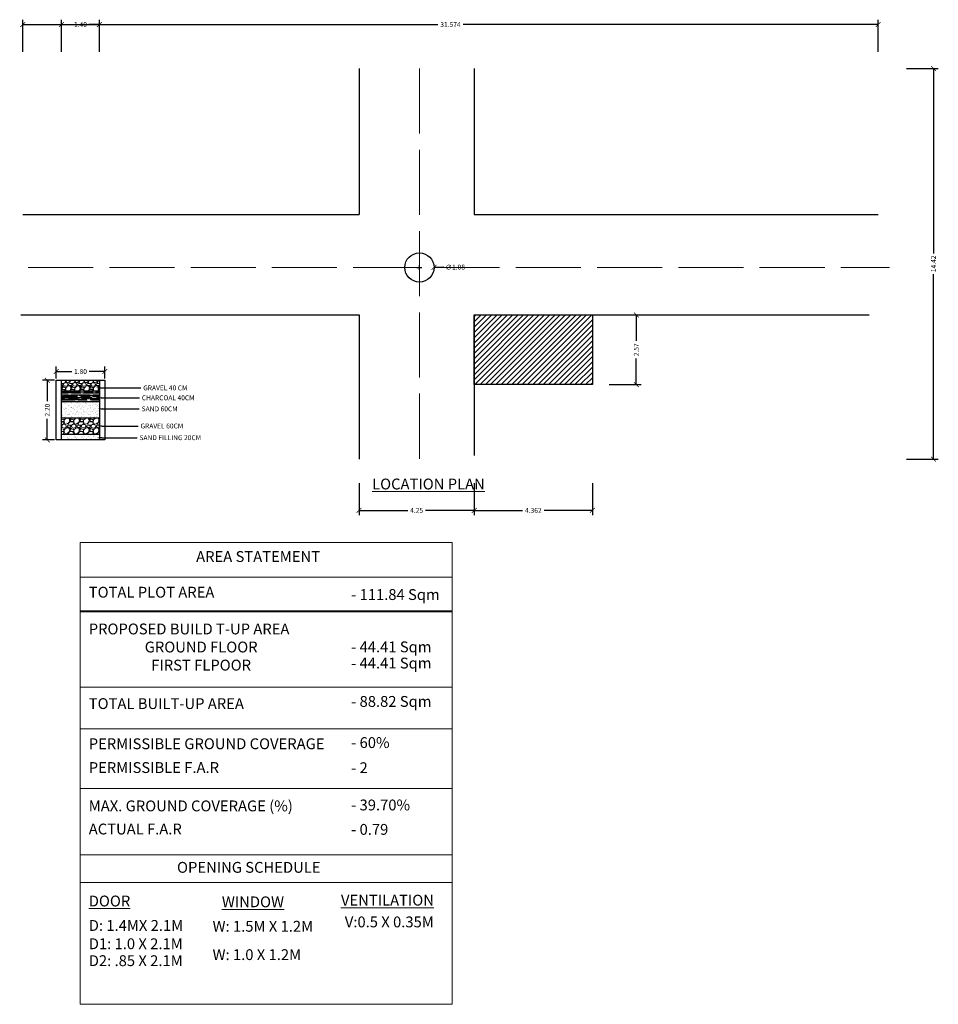
# Model space of a CAD drawing. Units: metres. Extents: x 6.8 to 74, y 0.6 to 37.
# Tile 5 of 5: x 40.1 to 74, y 0.6 to 37. Entities that reach past the tile are written whole.
import ezdxf
from ezdxf import colors
from ezdxf.entities.mleader import LeaderData, LeaderLine
from ezdxf.math import Vec2, Vec3

# ---------------------------------------------------------------- set-up
doc = ezdxf.new("R2010")
doc.units = ezdxf.units.M
doc.header["$LTSCALE"] = 0.2
doc.header["$MEASUREMENT"] = 0
doc.linetypes.add('ACAD_ISO02W100', pattern=[15, 12, -3])
for name, color, linetype, lineweight in [('A-ANNO-DIMS', 2, 'Continuous', 18), ('A-ANNO-SCHD', 7, 'Continuous', 18), ('A-ANNO-TEXT', 7, 'Continuous', 18), ('A-DETL', 7, 'Continuous', 25), ('A-DETL-PATT', 252, 'Continuous', 13), ('A-SCHD-TEXT', 7, 'Continuous', 18), ('C-PROP', 3, 'Continuous', 30), ('C-ROAD', 7, 'Continuous', 25), ('C-ROAD-CNTR', 1, 'ACAD_ISO02W100', 13), ('C-SITE-PATT', 252, 'Continuous', 13)]:
    doc.layers.add(name, color=color, linetype=linetype, lineweight=lineweight)
doc.styles.get("Standard").update_dxf_attribs({"font": 'arial.ttf'})
doc.dimstyles.get("Standard").update_dxf_attribs({"dimtxt": 0.18, "dimasz": 0.18, "dimexe": 0.18, "dimexo": 0.0625, "dimgap": 0.09, "dimtad": 0, "dimzin": 0, "dimdsep": 46, "dimtxsty": 'Standard', "dimblk": 'ARCHTICK', "dimcen": 0.09, "dimadec": 0, "dimazin": 0, "dimtfac": 1, "dimtofl": 0, "dimtmove": 0, "dimatfit": 3, "dimfxl": 1, "dimfxlon": 1, "dimtolj": 1, "dimtzin": 0, "dimarcsym": 0})
pattern_1 = [(37.5, (-6.10384, 6.83686), (-0.00548042, 0.16763367), [0, -0.13224, 0, -0.1479, 0, -0.141375]), (7.5, (-6.10384, 6.83686), (0.1539706, 0.2455267), [0, -0.07134, 0, -0.11919, 0, -0.045675]), (327.5, (-6.21085, 6.83686), (0.27093034, 0.00049234), [0, -0.0435, 0, -0.1566, 0, -0.20445]), (317.5, (-6.21085, 6.83686), (0.261533, 0.0763578), [0, -0.02175, 0, -0.10266, 0, -0.11745])]

# ---------------------------------------------------------------- blocks, each defined once
blk = doc.blocks.new('_ArchTick')
at = {"color": 0, "linetype": 'ByBlock', "const_width": 0.15}
blk.add_lwpolyline([(-0.5, -0.5), (0.5, 0.5)], dxfattribs=at)
blk = doc.blocks.new('*D14')
at = {"layer": 'A-ANNO-DIMS', "color": 0, "lineweight": -2, "ltscale": 0.9, "transparency": 16777216}
for p, q in [((41.484, 23.715), (41.484, 24.158)), ((43.284, 23.715), (43.284, 24.158)), ((41.484, 23.978), (42.069, 23.978)), ((43.284, 23.978), (42.699, 23.978))]:
    blk.add_line(p, q, dxfattribs=at)
at = {"layer": 'Defpoints', "color": 0, "ltscale": 0.9, "transparency": 16777216}
for p in [(41.484, 23.653), (43.284, 23.978), (43.284, 23.653)]:
    blk.add_point(p, dxfattribs=at)
at = {"layer": 'A-ANNO-DIMS', "color": 0, "lineweight": -2, "ltscale": 0.9, "transparency": 16777216, "xscale": 0.18, "yscale": 0.18, "zscale": 0.18, "rotation": 180}
blk.add_blockref('_ArchTick', (41.484, 23.978), dxfattribs=at)
at = {"layer": 'A-ANNO-DIMS', "color": 0, "lineweight": -2, "ltscale": 0.9, "transparency": 16777216, "xscale": 0.18, "yscale": 0.18, "zscale": 0.18}
blk.add_blockref('_ArchTick', (43.284, 23.978), dxfattribs=at)
at = {"layer": 'A-ANNO-DIMS', "color": 0, "ltscale": 0.9, "transparency": 16777216, "insert": (42.384, 23.978), "char_height": 0.18, "attachment_point": 5}
blk.add_mtext('\\A1;1.80', dxfattribs=at)
blk = doc.blocks.new('*D15')
at = {"layer": 'A-ANNO-DIMS', "color": 0, "lineweight": -2, "ltscale": 0.9, "transparency": 16777216}
for p, q in [((41.421, 23.653), (40.981, 23.653)), ((41.161, 23.653), (41.161, 22.878)), ((41.161, 21.453), (41.161, 22.228)), ((41.421, 21.453), (40.981, 21.453))]:
    blk.add_line(p, q, dxfattribs=at)
at = {"layer": 'Defpoints', "color": 0, "ltscale": 0.9, "transparency": 16777216}
for p in [(41.484, 23.653), (41.161, 21.453), (41.484, 21.453)]:
    blk.add_point(p, dxfattribs=at)
at = {"layer": 'A-ANNO-DIMS', "color": 0, "lineweight": -2, "ltscale": 0.9, "transparency": 16777216, "xscale": 0.18, "yscale": 0.18, "zscale": 0.18}
for p, rotation in [((41.161, 23.653), 90), ((41.161, 21.453), 270)]:
    blk.add_blockref('_ArchTick', p, dxfattribs=dict(at, rotation=rotation))
at = {"layer": 'A-ANNO-DIMS', "color": 0, "ltscale": 0.9, "transparency": 16777216, "insert": (41.161, 22.553), "char_height": 0.18, "attachment_point": 5, "rotation": 90}
blk.add_mtext('\\A1;2.20', dxfattribs=at)
blk = doc.blocks.new('*D60')
at = {"layer": 'A-ANNO-DIMS', "color": 0, "lineweight": -2, "ltscale": 0.9, "transparency": 16777216}
for p, q in [((52.667, 19.852), (52.667, 18.672)), ((56.917, 19.852), (56.917, 18.672)), ((52.667, 18.852), (54.464, 18.852)), ((56.917, 18.852), (55.12, 18.852))]:
    blk.add_line(p, q, dxfattribs=at)
at = {"layer": 'Defpoints', "color": 0, "ltscale": 0.9, "transparency": 16777216}
for p in [(52.667, 26.063), (56.917, 26.063), (56.917, 18.852)]:
    blk.add_point(p, dxfattribs=at)
at = {"layer": 'A-ANNO-DIMS', "color": 0, "lineweight": -2, "ltscale": 0.9, "transparency": 16777216, "xscale": 0.18, "yscale": 0.18, "zscale": 0.18, "rotation": 180}
blk.add_blockref('_ArchTick', (52.667, 18.852), dxfattribs=at)
at = {"layer": 'A-ANNO-DIMS', "color": 0, "lineweight": -2, "ltscale": 0.9, "transparency": 16777216, "xscale": 0.18, "yscale": 0.18, "zscale": 0.18}
blk.add_blockref('_ArchTick', (56.917, 18.852), dxfattribs=at)
at = {"layer": 'A-ANNO-DIMS', "color": 0, "ltscale": 0.9, "transparency": 16777216, "insert": (54.792, 18.852), "char_height": 0.18, "attachment_point": 5}
blk.add_mtext('\\A1;4.25', dxfattribs=at)
blk = doc.blocks.new('*D61')
at = {"layer": 'A-ANNO-DIMS', "color": 0, "lineweight": -2, "ltscale": 0.9, "transparency": 16777216}
for p, q in [((39.567, 29.769), (38.387, 29.769)), ((38.567, 29.769), (38.567, 28.31)), ((38.567, 26.063), (38.567, 27.523)), ((39.567, 26.063), (38.387, 26.063))]:
    blk.add_line(p, q, dxfattribs=at)
at = {"layer": 'Defpoints', "color": 0, "ltscale": 0.9, "transparency": 16777216}
for p in [(38.567, 29.769), (52.667, 29.769), (52.667, 26.063)]:
    blk.add_point(p, dxfattribs=at)
at = {"layer": 'A-ANNO-DIMS', "color": 0, "lineweight": -2, "ltscale": 0.9, "transparency": 16777216, "xscale": 0.18, "yscale": 0.18, "zscale": 0.18}
for p, rotation in [((38.567, 29.769), 90), ((38.567, 26.063), 270)]:
    blk.add_blockref('_ArchTick', p, dxfattribs=dict(at, rotation=rotation))
at = {"layer": 'A-ANNO-DIMS', "color": 0, "ltscale": 0.9, "transparency": 16777216, "insert": (38.567, 27.916), "char_height": 0.18, "attachment_point": 5, "rotation": 90}
blk.add_mtext('\\A1;3.706', dxfattribs=at)
blk = doc.blocks.new('*D62')
at = {"layer": 'A-ANNO-DIMS', "color": 0, "lineweight": -2, "ltscale": 0.9, "transparency": 16777216}
for p, q in [((56.917, 19.852), (56.917, 18.672)), ((61.279, 19.852), (61.279, 18.672)), ((56.917, 18.852), (58.702, 18.852)), ((61.279, 18.852), (59.495, 18.852))]:
    blk.add_line(p, q, dxfattribs=at)
at = {"layer": 'Defpoints', "color": 0, "ltscale": 0.9, "transparency": 16777216}
for p in [(56.917, 23.493), (61.279, 23.493), (61.279, 18.852)]:
    blk.add_point(p, dxfattribs=at)
at = {"layer": 'A-ANNO-DIMS', "color": 0, "lineweight": -2, "ltscale": 0.9, "transparency": 16777216, "xscale": 0.18, "yscale": 0.18, "zscale": 0.18, "rotation": 180}
blk.add_blockref('_ArchTick', (56.917, 18.852), dxfattribs=at)
at = {"layer": 'A-ANNO-DIMS', "color": 0, "lineweight": -2, "ltscale": 0.9, "transparency": 16777216, "xscale": 0.18, "yscale": 0.18, "zscale": 0.18}
blk.add_blockref('_ArchTick', (61.279, 18.852), dxfattribs=at)
at = {"layer": 'A-ANNO-DIMS', "color": 0, "ltscale": 0.9, "transparency": 16777216, "insert": (59.098, 18.852), "char_height": 0.18, "attachment_point": 5}
blk.add_mtext('\\A1;4.362', dxfattribs=at)
blk = doc.blocks.new('*D63')
at = {"layer": 'A-ANNO-DIMS', "color": 0, "lineweight": -2, "ltscale": 0.9, "transparency": 16777216}
for p, q in [((61.898, 26.063), (63.078, 26.063)), ((62.898, 26.063), (62.898, 25.103)), ((62.898, 23.493), (62.898, 24.453)), ((61.898, 23.493), (63.078, 23.493))]:
    blk.add_line(p, q, dxfattribs=at)
at = {"layer": 'Defpoints', "color": 0, "ltscale": 0.9, "transparency": 16777216}
for p in [(61.279, 26.063), (61.279, 23.493), (62.898, 23.493)]:
    blk.add_point(p, dxfattribs=at)
at = {"layer": 'A-ANNO-DIMS', "color": 0, "lineweight": -2, "ltscale": 0.9, "transparency": 16777216, "xscale": 0.18, "yscale": 0.18, "zscale": 0.18}
for p, rotation in [((62.898, 26.063), 90), ((62.898, 23.493), 270)]:
    blk.add_blockref('_ArchTick', p, dxfattribs=dict(at, rotation=rotation))
at = {"layer": 'A-ANNO-DIMS', "color": 0, "ltscale": 0.9, "transparency": 16777216, "insert": (62.898, 24.778), "char_height": 0.18, "attachment_point": 5, "rotation": 90}
blk.add_mtext('\\A1;2.57', dxfattribs=at)
blk = doc.blocks.new('*D64')
at = {"layer": 'A-ANNO-DIMS', "color": 0, "lineweight": -2, "ltscale": 0.9, "transparency": 16777216}
for p, q in [((41.683909, 35.779105), (41.683909, 36.959105)), ((41.683909, 36.779105), (42.068909, 36.779105)), ((43.083909, 36.779105), (42.698909, 36.779105)), ((43.083909, 35.779105), (43.083909, 36.959105))]:
    blk.add_line(p, q, dxfattribs=at)
at = {"layer": 'Defpoints', "color": 0, "ltscale": 0.9, "transparency": 16777216}
for p in [(43.083909, 36.779105), (41.683909, 23.652882), (43.083909, 23.652882)]:
    blk.add_point(p, dxfattribs=at)
at = {"layer": 'A-ANNO-DIMS', "color": 0, "lineweight": -2, "ltscale": 0.9, "transparency": 16777216, "xscale": 0.18, "yscale": 0.18, "zscale": 0.18, "rotation": 180}
blk.add_blockref('_ArchTick', (41.683909, 36.779105), dxfattribs=at)
at = {"layer": 'A-ANNO-DIMS', "color": 0, "lineweight": -2, "ltscale": 0.9, "transparency": 16777216, "xscale": 0.18, "yscale": 0.18, "zscale": 0.18}
blk.add_blockref('_ArchTick', (43.083909, 36.779105), dxfattribs=at)
at = {"layer": 'A-ANNO-DIMS', "color": 0, "ltscale": 0.9, "transparency": 16777216, "insert": (42.383909, 36.779105), "char_height": 0.18, "attachment_point": 5}
blk.add_mtext('\\A1;1.40', dxfattribs=at)
blk = doc.blocks.new('*D75')
at = {"layer": 'A-ANNO-DIMS', "color": 0, "lineweight": -2, "ltscale": 0.9, "transparency": 16777216}
for p, q in [((40.253, 35.779), (40.253, 36.959)), ((40.253, 36.779), (55.577, 36.779)), ((71.827, 36.779), (56.504, 36.779)), ((71.827, 35.779), (71.827, 36.959))]:
    blk.add_line(p, q, dxfattribs=at)
at = {"layer": 'Defpoints', "color": 0, "ltscale": 0.9, "transparency": 16777216}
for p in [(71.827, 36.779), (40.253, 29.769), (71.827, 29.769)]:
    blk.add_point(p, dxfattribs=at)
at = {"layer": 'A-ANNO-DIMS', "color": 0, "lineweight": -2, "ltscale": 0.9, "transparency": 16777216, "xscale": 0.18, "yscale": 0.18, "zscale": 0.18, "rotation": 180}
blk.add_blockref('_ArchTick', (40.253, 36.779), dxfattribs=at)
at = {"layer": 'A-ANNO-DIMS', "color": 0, "lineweight": -2, "ltscale": 0.9, "transparency": 16777216, "xscale": 0.18, "yscale": 0.18, "zscale": 0.18}
blk.add_blockref('_ArchTick', (71.827, 36.779), dxfattribs=at)
at = {"layer": 'A-ANNO-DIMS', "color": 0, "ltscale": 0.9, "transparency": 16777216, "insert": (56.04, 36.779), "char_height": 0.18, "attachment_point": 5}
blk.add_mtext('\\A1;31.574', dxfattribs=at)
blk = doc.blocks.new('*D76')
at = {"layer": 'A-ANNO-DIMS', "color": 0, "lineweight": -2, "ltscale": 0.9, "transparency": 16777216}
for p, q in [((72.866, 35.16), (74.046, 35.16)), ((73.866, 35.16), (73.866, 28.334)), ((73.866, 20.74), (73.866, 27.566)), ((72.866, 20.74), (74.046, 20.74))]:
    blk.add_line(p, q, dxfattribs=at)
at = {"layer": 'Defpoints', "color": 0, "ltscale": 0.9, "transparency": 16777216}
for p in [(52.667, 35.16), (73.866, 35.16), (52.667, 20.74)]:
    blk.add_point(p, dxfattribs=at)
at = {"layer": 'A-ANNO-DIMS', "color": 0, "lineweight": -2, "ltscale": 0.9, "transparency": 16777216, "xscale": 0.18, "yscale": 0.18, "zscale": 0.18}
for p, rotation in [((73.866, 35.16), 90), ((73.866, 20.74), 270)]:
    blk.add_blockref('_ArchTick', p, dxfattribs=dict(at, rotation=rotation))
at = {"layer": 'A-ANNO-DIMS', "color": 0, "ltscale": 0.9, "transparency": 16777216, "insert": (73.866, 27.95), "char_height": 0.18, "attachment_point": 5, "rotation": 90}
blk.add_mtext('\\A1;14.42', dxfattribs=at)
blk = doc.blocks.new('*D77')
at = {"layer": 'A-ANNO-DIMS', "color": 0, "lineweight": -2, "ltscale": 0.9, "transparency": 16777216}
for p, q in [((54.803, 27.815), (54.983, 27.815)), ((54.893, 27.725), (54.893, 27.905)), ((55.793, 27.823), (55.433, 27.82))]:
    blk.add_line(p, q, dxfattribs=at)
at = {"layer": 'Defpoints', "color": 0, "ltscale": 0.9, "transparency": 16777216}
for p in [(54.354, 27.811), (55.433, 27.82)]:
    blk.add_point(p, dxfattribs=at)
at = {"layer": 'A-ANNO-DIMS', "color": 0, "lineweight": -2, "ltscale": 0.9, "transparency": 16777216, "xscale": 0.18, "yscale": 0.18, "zscale": 0.18, "rotation": 180.5010629486621}
blk.add_blockref('_ArchTick', (55.433, 27.82), dxfattribs=at)
at = {"layer": 'A-ANNO-DIMS', "color": 0, "ltscale": 0.9, "transparency": 16777216, "insert": (56.215, 27.827), "char_height": 0.18, "attachment_point": 5, "rotation": 0.5011}
blk.add_mtext('\\A1;∅1.08', dxfattribs=at)

msp = doc.modelspace()

# ---------------------------------------------------------------- hatches: boundary and pattern name
at = {"layer": 'A-DETL-PATT', "ltscale": 0.9}
h = msp.add_hatch(dxfattribs=at)
h.set_pattern_fill('GRAVEL', color=256, scale=0.34)
h.set_pattern_definition([(228.01279, (-5.85904, 7.176862), (-2.72, -3.06), [0.0457422, -4.52849]), (184.96974, (-5.88964, 7.142862), (4.08, 0.34), [0.0784951, -7.7710144]), (132.510447, (-5.96784, 7.136062), (3.4, -3.74), [0.055348, -5.479451]), (267.27369, (-6.10044, 7.051062), (0.34, 6.8), [0.071481, -7.0766097]), (292.833654, (-6.10384, 6.979662), (-1.7, 4.08), [0.0700927, -6.9391869]), (357.27369, (-6.07664, 6.915062), (-6.8, 0.34), [0.071481, -7.0766097]), (37.69424, (-6.00524, 6.911662), (-4.42, -3.4), [0.0945299, -9.3584485]), (72.255328, (-5.93044, 6.969462), (2.38, 7.48), [0.089246, -8.8353493]), (121.429566, (-5.90324, 7.054462), (-2.72, 4.42), [0.071723, -7.1005849]), (175.23636, (-5.94064, 7.115662), (3.74, -0.34), [0.0818829, -4.0122593]), (222.397438, (-6.02224, 7.122462), (-4.08, -3.74), [0.1058923, -10.4833475]), (138.814075, (-5.76384, 7.04766), (-2.38, 2.04), [0.0361423, -3.5781072]), (171.469234, (-5.79104, 7.071462), (4.42, -0.68), [0.0687606, -6.8073139]), (225, (-5.85904, 7.08166), (0, -0.34), [0.0480831, -0.4327495]), (203.19859, (-5.88284, 7.12246), (1.7, 0.68), [0.0258937, -2.5634691]), (291.80141, (-5.90664, 7.11226), (-0.34, 1.02), [0.036619, -1.794337]), (30.96376, (-5.89304, 7.07826), (1.02, 0.68), [0.0594759, -1.9230478]), (161.56505, (-5.84204, 7.10886), (0.68, -0.34), [0.043007, -1.0321675]), (16.38954, (-6.10384, 7.112262), (3.4, 1.02), [0.060248, -5.9645673]), (70.346176, (-6.04604, 7.129262), (-1.36, -3.74), [0.0505447, -5.0039186]), (293.19859, (-5.84204, 7.17686), (-0.68, 1.7), [0.051787, -2.5375758]), (343.61046, (-5.82164, 7.129262), (-3.4, 1.02), [0.060248, -5.9645673]), (339.443955, (-6.10384, 6.90146), (-1.7, 0.68), [0.0580992, -2.846862]), (294.77514, (-6.04944, 6.881062), (-1.7, 3.74), [0.0486805, -4.8193786]), (66.80141, (-5.83864, 6.83686), (0.68, 1.7), [0.051787, -2.5375758]), (17.354025, (-5.81824, 6.884462), (-4.42, -1.36), [0.0569945, -5.642444]), (69.443955, (-6.00524, 6.83686), (-0.68, -1.7), [0.0290496, -2.8759117]), (101.30993, (-5.85904, 6.83686), (-0.34, 1.36), [0.0173366, -1.71633]), (165.96376, (-5.86244, 6.85386), (1.02, -0.34), [0.0700927, -1.3317632]), (186.009006, (-5.93044, 6.870862), (3.4, 0.34), [0.064957, -6.4307339]), (303.69007, (-5.89304, 7.04766), (-0.34, 0.68), [0.0490355, -1.176852]), (353.157227, (-5.86584, 7.006862), (5.78, -0.68), [0.08561, -8.4753713]), (60.945396, (-5.78084, 6.99666), (-1.36, -2.38), [0.035005, -3.4655092]), (90, (-5.76384, 7.02726), (-0.34, 0.34), [0.0204, -0.3196]), (120.256437, (-5.93724, 6.881062), (1.36, -2.38), [0.0472342, -4.6761968]), (48.01279, (-5.96104, 6.921862), (2.72, 3.06), [0.0914845, -4.4827477]), (0, (-5.89984, 6.98986), (0.34, 0.34), [0.0884, -0.2516]), (325.304846, (-5.81144, 6.989862), (3.4, -2.38), [0.0537588, -5.3221133]), (254.0546, (-5.76724, 6.95926), (-0.34, -1.36), [0.0495047, -2.4257327]), (207.645975, (-5.78084, 6.911662), (-6.46, -3.4), [0.0806021, -7.9796212]), (175.42608, (-5.85224, 6.874262), (-4.42, 0.34), [0.0852717, -8.441885])])
h.paths.add_polyline_path([(41.6839, 23.6529), (41.6839, 23.2529), (43.0839, 23.2529), (43.0839, 23.6529)])
h = msp.add_hatch(dxfattribs=at)
h.set_pattern_fill('AR-RROOF', color=256, scale=0.087)
h.set_pattern_definition([(0, (-6.10384, 6.83686), (0.1914, 0.087), [1.305, -0.174, 0.435, -0.087]), (0, (-5.98813, 6.88036), (-0.087, 0.11571), [0.261, -0.02871, 0.522, -0.06525]), (0, (-6.06034, 6.91081), (0.4524, 0.05829), [0.696, -0.1218, 0.348, -0.087])])
h.paths.add_polyline_path([(43.0839, 22.8529), (43.0839, 23.2529), (41.6839, 23.2529), (41.6839, 22.8529)])
h = msp.add_hatch(dxfattribs=at)
h.set_pattern_fill('AR-SAND', color=256, scale=0.087)
h.set_pattern_definition(pattern_1)
h.paths.add_polyline_path([(41.6839, 22.8529), (41.6839, 22.2529), (43.0839, 22.2529), (43.0839, 22.8529)])
h = msp.add_hatch(dxfattribs=at)
h.set_pattern_fill('GRAVEL', color=256, scale=0.36)
h.set_pattern_definition([(228.01279, (-5.84464, 7.196862), (-2.88, -3.24), [0.048433, -4.7948717]), (184.96974, (-5.87704, 7.160862), (4.32, 0.36), [0.0831125, -8.228133]), (132.510447, (-5.95984, 7.153662), (3.6, -3.96), [0.0586037, -5.8017717]), (267.27369, (-6.10024, 7.063662), (0.36, 7.2), [0.0756857, -7.492881]), (292.833654, (-6.10384, 6.988062), (-1.8, 4.32), [0.0742158, -7.3473743]), (357.27369, (-6.07504, 6.919662), (-7.2, 0.36), [0.0756857, -7.492881]), (37.69424, (-5.99944, 6.916062), (-4.68, -3.6), [0.1000904, -9.9089455]), (72.255328, (-5.92024, 6.977262), (2.52, 7.92), [0.0944957, -9.3550757]), (121.429566, (-5.89144, 7.067262), (-2.88, 4.68), [0.075942, -7.5182663]), (175.23636, (-5.93104, 7.132062), (3.96, -0.36), [0.0866995, -4.2482745]), (222.397438, (-6.01744, 7.139262), (-4.32, -3.96), [0.1121213, -11.100015]), (138.814075, (-5.74384, 7.06006), (-2.52, 2.16), [0.0382684, -3.7885841]), (171.469234, (-5.77264, 7.085262), (4.68, -0.72), [0.0728053, -7.207744]), (225, (-5.84464, 7.09606), (0, -0.36), [0.0509116, -0.4582053]), (203.19859, (-5.86984, 7.13926), (1.8, 0.72), [0.027417, -2.7142614]), (291.80141, (-5.89504, 7.12846), (-0.36, 1.08), [0.038773, -1.8998863]), (30.96376, (-5.88064, 7.09246), (1.08, 0.72), [0.0629744, -2.0361682]), (161.56505, (-5.82664, 7.12486), (0.72, -0.36), [0.0455368, -1.0928832]), (16.38954, (-6.10384, 7.128462), (3.6, 1.08), [0.063792, -6.3154243]), (70.346176, (-6.04264, 7.146462), (-1.44, -3.96), [0.053518, -5.2982668]), (293.19859, (-5.82664, 7.19686), (-0.72, 1.8), [0.0548334, -2.686845]), (343.61046, (-5.80504, 7.146462), (-3.6, 1.08), [0.063792, -6.3154243]), (339.443955, (-6.10384, 6.90526), (-1.8, 0.72), [0.0615168, -3.0143245]), (294.77514, (-6.04624, 6.883662), (-1.8, 3.96), [0.051544, -5.1028715]), (66.80141, (-5.82304, 6.83686), (0.72, 1.8), [0.0548334, -2.686845]), (17.354025, (-5.80144, 6.887262), (-4.68, -1.44), [0.0603472, -5.9743525]), (69.443955, (-5.99944, 6.83686), (-0.72, -1.8), [0.0307584, -3.045083]), (101.30993, (-5.84464, 6.83686), (-0.36, 1.44), [0.0183564, -1.8172906]), (165.96376, (-5.84824, 6.85486), (1.08, -0.36), [0.0742158, -1.4101022]), (186.009006, (-5.92024, 6.872862), (3.6, 0.36), [0.068778, -6.8090123]), (303.69007, (-5.88064, 7.06006), (-0.36, 0.72), [0.05192, -1.2460785]), (353.157227, (-5.85184, 7.016862), (6.12, -0.72), [0.0906458, -8.9739225]), (60.945396, (-5.76184, 7.00606), (-1.44, -2.52), [0.0370642, -3.6693627]), (90, (-5.74384, 7.03846), (-0.36, 0.36), [0.0216, -0.3384]), (120.25644, (-5.92744, 6.883662), (1.44, -2.52), [0.0500126, -4.9512672]), (48.01279, (-5.95264, 6.926862), (2.88, 3.24), [0.096866, -4.7464387]), (0, (-5.88784, 6.99886), (0.36, 0.36), [0.0936, -0.2664]), (325.304846, (-5.79424, 6.998862), (3.6, -2.52), [0.056921, -5.6351787]), (254.0546, (-5.74744, 6.96646), (-0.36, -1.44), [0.0524167, -2.5684228]), (207.645975, (-5.76184, 6.916062), (-6.84, -3.6), [0.0853434, -8.4490107]), (175.42608, (-5.83744, 6.876462), (-4.68, 0.36), [0.0902876, -8.9384664])])
h.paths.add_polyline_path([(43.0839, 21.6529), (43.0839, 22.2529), (41.6839, 22.2529), (41.6839, 21.6529)])
h = msp.add_hatch(dxfattribs=at)
h.set_pattern_fill('AR-SAND', color=256, scale=0.087)
h.set_pattern_definition(pattern_1)
h.paths.add_polyline_path([(43.0839, 21.4529), (43.0839, 21.6529), (41.6839, 21.6529), (41.6839, 21.4529)])
at = {"layer": 'C-SITE-PATT', "ltscale": 0.9}
h = msp.add_hatch(dxfattribs=at)
h.set_pattern_fill('ANSI31', color=256, scale=1.1)
h.paths.add_polyline_path([(61.2791, 26.0633), (56.9174, 26.0633), (56.9174, 23.4929), (61.2791, 23.4929)])

# ---------------------------------------------------------------- linework, layer by layer
at = {"layer": 'A-ANNO-SCHD', "ltscale": 0.9}
for p, q in [((42.3695, 16.3885), (56.0997, 16.3885)), ((42.3695, 15.1397), (56.0997, 15.1397)), ((42.3695, 15.1297), (56.0997, 15.1297)), ((42.3695, 15.1197), (56.0997, 15.1197)), ((42.3695, 15.1097), (56.0997, 15.1097)), ((42.3695, 12.326), (56.0997, 12.326)), ((42.3695, 10.7916), (56.0997, 10.7916)), ((42.3695, 8.5874), (56.0997, 8.5874)), ((42.3695, 6.1366), (56.0997, 6.1366)), ((42.3695, 5.1183), (56.0997, 5.1183))]:
    msp.add_line(p, q, dxfattribs=at)
msp.add_lwpolyline([(42.3695, 17.6615), (56.0997, 17.6615), (56.0997, 0.6263), (42.3695, 0.6263)], close=True, dxfattribs=at)
at = {"layer": 'A-DETL', "ltscale": 0.9}
for p, q in [((41.4839, 23.6529), (43.2839, 23.6529)), ((41.4839, 21.4529), (41.4839, 23.6529)), ((41.6839, 21.4529), (41.6839, 23.6529)), ((43.0839, 23.6529), (43.0839, 21.4529)), ((43.2839, 23.6529), (43.2839, 21.4529)), ((43.0839, 23.2529), (41.6839, 23.2529)), ((43.0839, 22.8529), (41.6839, 22.8529)), ((43.0839, 22.2529), (41.6839, 22.2529)), ((43.2839, 21.4529), (41.4839, 21.4529)), ((43.0839, 21.6529), (41.6839, 21.6529))]:
    msp.add_line(p, q, dxfattribs=at)
at = {"layer": 'C-PROP', "ltscale": 0.9}
msp.add_lwpolyline([(56.9174, 26.0633), (61.2791, 26.0633), (61.2791, 23.4929), (56.9174, 23.4929)], close=True, dxfattribs=at)
at = {"layer": 'C-ROAD'}
for p, q in [((52.667, 35.1601), (52.667, 29.7694)), ((56.9174, 35.1601), (56.9174, 29.7694)), ((40.2531, 29.7694), (52.667, 29.7694)), ((56.9174, 29.7694), (71.8275, 29.7694)), ((40.1857, 26.0633), (52.667, 26.0633)), ((52.667, 26.0633), (52.667, 20.74)), ((56.9174, 26.0633), (56.9174, 20.8748)), ((56.9174, 26.0633), (71.4901, 26.0633))]:
    msp.add_line(p, q, dxfattribs=at)
msp.add_circle((54.8934, 27.8153), 0.5397, dxfattribs=at)
at = {"layer": 'C-ROAD-CNTR'}
for p, q in [((54.8934, 35.1601), (54.8934, 20.4705)), ((40.4522, 27.8153), (72.2468, 27.8153))]:
    msp.add_line(p, q, dxfattribs=at)

# ---------------------------------------------------------------- texts
at = {"layer": 'A-ANNO-TEXT', "insert": (53.1485, 20.0251), "char_height": 0.4, "attachment_point": 1}
msp.add_mtext_dynamic_manual_height_columns('{\\LLOCATION PLAN}', width=7.004508, gutter_width=1, heights=[0], dxfattribs=at)
at = {"layer": 'A-SCHD-TEXT', "char_height": 0.4, "attachment_point": 1}
for s, width, heights, insert in [('{\\fArial|b1|i0|c0|p34;AREA STATEMENT}', 7.004508, [0], (46.6538, 17.3488)), ('\\pxt8;TOTAL PLOT AREA', 7.004508, [0], (42.69, 16.033)), ('\\pxt8;{\\fArial|b1|i0|c0|p34;- }111.84 Sqm', 7.004508, [0], (52.3737, 15.9458)), ('\\pxt8;PROPOSED BUILD T-UP AREA\\P\\pqc;GROUND FLOOR \\PFIRST FLPOOR', 8.29728, [0], (42.69, 14.6767)), ('\\pxt8;{\\fArial|b1|i0|c0|p34;- }44.41 Sqm', 7.004508, [0], (52.3737, 14.0155)), ('\\pxt8;{\\fArial|b1|i0|c0|p34;- }44.41 Sqm', 7.004508, [0], (52.3737, 13.4178)), ('\\pxt8;{\\fArial|b1|i0|c0|p34;- }88.82 Sqm', 7.004508, [0], (52.3737, 12.0028)), ('\\pxt8;TOTAL BUILT-UP AREA', 7.004508, [0], (42.69, 11.9228)), ('PERMISSIBLE GROUND COVERAGE', 9.901275, [0], (42.69, 10.4403)), ('\\pxt8;{\\fArial|b1|i0|c0|p34;- }60%', 7.004508, [0], (52.3737, 10.484)), ('PERMISSIBLE F.A.R', 9.901275, [0], (42.69, 9.5624)), ('{\\fArial|b1|i0|c0|p34;- }2', 7.004508, [0], (52.3737, 9.5557)), ('MAX. GROUND COVERAGE (%)', 9.901275, [0], (42.69, 8.1472)), ('{\\fArial|b1|i0|c0|p34;- }39.70%', 7.004508, [0], (52.3737, 8.1818)), ('ACTUAL F.A.R', 9.901275, [0], (42.69, 7.2934)), ('{\\fArial|b1|i0|c0|p34;- }0.79', 7.004508, [0], (52.3737, 7.2814)), ('{\\fArial|b1|i0|c0|p34;OPENING SCHEDULE}', 9.901275, [0], (45.9479, 5.8797)), ('{\\fArial|b1|i0|c0|p34;\\LDOOR}', 2.486776, [0], (42.69, 4.6378)), ('{\\fArial|b1|i0|c0|p34;\\LWINDOW}', 2.486776, [0], (47.6036, 4.6066)), ('{\\fArial|b1|i0|c0|p34;\\LVENTILATION}', 2.486776, [0], (51.9992, 4.6691)), ('D: 1.4MX 2.1M', 4.223083, [0.4136], (42.69, 3.7363)), ('W: 1.5M X 1.2M', 4.223083, [0.4136], (47.2595, 3.705)), ('V:0.5 X 0.35M', 4.223083, [0.4136], (52.1412, 3.8665)), ('D1: 1.0 X 2.1M', 4.801851, [0], (42.69, 3.0609)), ('W: 1.0 X 1.2M', 4.223083, [0.4136], (47.2595, 2.6586)), ('D2: .85 X 2.1M', 4.301295, [0], (42.69, 2.4359))]:
    msp.add_mtext_dynamic_manual_height_columns(s, width=width, gutter_width=1, heights=heights, dxfattribs=dict(at, insert=insert))

# ---------------------------------------------------------------- dimensions: what is measured, and where the dimension line sits
at = {"layer": 'A-ANNO-DIMS', "ltscale": 0.9}
for base, p1, p2, override, picture, middle in [((71.8275, 36.7791), (40.2531, 29.7694), (71.8275, 29.7694), {"dimdec": 3, "dimlfac": 1, "dimrnd": 0, "dimzin": 0, "dimdsep": 46, "dimlunit": 2}, '*D75', (56.0403, 36.7791)), ((43.0839, 36.7791), (41.6839, 23.6529), (43.0839, 23.6529), {"dimdec": 2, "dimlfac": 1, "dimrnd": 0, "dimzin": 0, "dimdsep": 46, "dimlunit": 2}, '*D64', (42.3839, 36.7791)), ((56.9174, 18.8515), (52.667, 26.0633), (56.9174, 26.0633), {"dimdec": 2, "dimlfac": 1, "dimrnd": 0, "dimzin": 0, "dimdsep": 46, "dimlunit": 2}, '*D60', (54.7922, 18.8515)), ((43.2839, 23.9785), (41.4839, 23.6529), (43.2839, 23.6529), {"dimclrd": 0, "dimclre": 0, "dimclrt": 0}, '*D14', (42.3839, 23.9785)), ((61.2791, 18.8515), (56.9174, 23.4929), (61.2791, 23.4929), {"dimdec": 3, "dimlfac": 1, "dimrnd": 0, "dimzin": 0, "dimdsep": 46, "dimlunit": 2}, '*D62', (59.0982, 18.8515))]:
    dim = msp.add_linear_dim(base=base, p1=p1, p2=p2, dimstyle='Standard', override=override, dxfattribs=at)
    dim.commit()
    dim.dimension.update_dxf_attribs({"geometry": picture, "text_midpoint": middle})
for base, p1, p2, angle, override, picture, middle in [((73.8658, 35.1601), (52.667, 20.74), (52.667, 35.1601), 90, {"dimdec": 2, "dimlfac": 1, "dimrnd": 0, "dimzin": 0, "dimdsep": 46, "dimlunit": 2}, '*D76', (73.8658, 27.9501)), ((38.5667, 29.7694), (52.667, 26.0633), (52.667, 29.7694), 90, {"dimdec": 3, "dimlfac": 1, "dimrnd": 0, "dimzin": 0, "dimdsep": 46, "dimlunit": 2}, '*D61', (38.5667, 27.9164)), ((62.8981, 23.4929), (61.2791, 26.0633), (61.2791, 23.4929), 270, {"dimdec": 2, "dimlfac": 1, "dimrnd": 0, "dimzin": 0, "dimdsep": 46, "dimlunit": 2}, '*D63', (62.8981, 24.7781)), ((41.161, 21.4529), (41.4839, 23.6529), (41.4839, 21.4529), 90, {"dimclrd": 0, "dimclre": 0, "dimclrt": 0}, '*D15', (41.161, 22.5529))]:
    dim = msp.add_linear_dim(base=base, p1=p1, p2=p2, angle=angle, dimstyle='Standard', override=override, dxfattribs=at)
    dim.commit()
    dim.dimension.update_dxf_attribs({"geometry": picture, "text_midpoint": middle})
dim = msp.add_diameter_dim_2p(p1=(54.3537, 27.8106), p2=(55.4331, 27.82), dimstyle='Standard', override={"dimdec": 2, "dimlfac": 1, "dimrnd": 0, "dimzin": 0, "dimdsep": 46, "dimlunit": 2}, dxfattribs=at)
dim.commit()
dim.dimension.update_dxf_attribs({"geometry": '*D77', "text_midpoint": (56.2149, 27.8269), "dimtype": 163})

# ---------------------------------------------------------------- leaders
at = {"layer": 'A-ANNO-TEXT', "ltscale": 0.9}
ml = msp.add_multileader_mtext('Standard', dxfattribs=at)
ml.set_content('GRAVEL 40 CM ', color=256)
ml.set_leader_properties()
ml.build(insert=Vec2(0, 0))
ml.multileader.update_dxf_attribs({"dogleg_length": 0.36, "arrow_head_size": 0.18})
ctx = ml.context
ctx.base_point, ctx.char_height, ctx.arrow_head_size, ctx.landing_gap_size, ctx.plane_origin = Vec3(44.6086, 23.37), 0.18, 0.18, 0.09, Vec3(42.9428, 23.37)
notes = []
notes.append((ctx, [(0, (1, 1, 0), (44.2486, 23.37), (1, 0), 0.36, [(0, [(42.9428, 23.37)], 0, [])])]))
ctx.mtext.insert, ctx.mtext.flow_direction = Vec3(44.6986, 23.4616), 5
ml = msp.add_multileader_mtext('Standard', dxfattribs=at)
ml.set_content('CHARCOAL 40CM', color=256)
ml.set_leader_properties()
ml.build(insert=Vec2(0, 0))
ml.multileader.update_dxf_attribs({"dogleg_length": 0.36, "arrow_head_size": 0.18})
ctx = ml.context
ctx.base_point, ctx.char_height, ctx.arrow_head_size, ctx.landing_gap_size, ctx.plane_origin = Vec3(44.5584, 23.0039), 0.18, 0.18, 0.09, Vec3(42.9981, 23.0039)
notes.append((ctx, [(0, (1, 1, 0), (44.1984, 23.0039), (1, 0), 0.36, [(0, [(42.9981, 23.0039)], 0, [])])]))
ctx.mtext.insert, ctx.mtext.flow_direction = Vec3(44.6484, 23.0954), 5
ml = msp.add_multileader_mtext('Standard', dxfattribs=at)
ml.set_content('SAND 60CM', color=256)
ml.set_leader_properties()
ml.build(insert=Vec2(0, 0))
ml.multileader.update_dxf_attribs({"dogleg_length": 0.36, "arrow_head_size": 0.18})
ctx = ml.context
ctx.base_point, ctx.char_height, ctx.arrow_head_size, ctx.landing_gap_size, ctx.plane_origin = Vec3(44.5535, 22.5965), 0.18, 0.18, 0.09, Vec3(43.0133, 22.5965)
notes.append((ctx, [(0, (1, 1, 0), (44.1935, 22.5965), (1, 0), 0.36, [(0, [(43.0133, 22.5965)], 0, [])])]))
ctx.mtext.insert, ctx.mtext.flow_direction = Vec3(44.6435, 22.688), 5
ml = msp.add_multileader_mtext('Standard', dxfattribs=at)
ml.set_content('GRAVEL 60CM', color=256)
ml.set_leader_properties()
ml.build(insert=Vec2(0, 0))
ml.multileader.update_dxf_attribs({"dogleg_length": 0.36, "arrow_head_size": 0.18})
ctx = ml.context
ctx.base_point, ctx.char_height, ctx.arrow_head_size, ctx.landing_gap_size, ctx.plane_origin = Vec3(44.5083, 21.9645), 0.18, 0.18, 0.09, Vec3(43.0032, 21.9645)
notes.append((ctx, [(0, (1, 1, 0), (44.1483, 21.9645), (1, 0), 0.36, [(0, [(43.0032, 21.9645)], 0, [])])]))
ctx.mtext.insert, ctx.mtext.flow_direction = Vec3(44.5983, 22.056), 5
ml = msp.add_multileader_mtext('Standard', dxfattribs=at)
ml.set_content('SAND FILLING 20CM', color=256)
ml.set_leader_properties()
ml.build(insert=Vec2(0, 0))
ml.multileader.update_dxf_attribs({"dogleg_length": 0.36, "arrow_head_size": 0.18})
ctx = ml.context
ctx.base_point, ctx.char_height, ctx.arrow_head_size, ctx.landing_gap_size, ctx.plane_origin = Vec3(44.4731, 21.5331), 0.18, 0.18, 0.09, Vec3(42.9932, 21.5331)
notes.append((ctx, [(0, (1, 1, 0), (44.1131, 21.5331), (1, 0), 0.36, [(0, [(42.9932, 21.5331)], 0, [])])]))
ctx.mtext.insert, ctx.mtext.flow_direction = Vec3(44.5631, 21.6247), 5
for ctx, leaders in notes:
    for number, flags, end, landing, length, lines in leaders:
        leader = LeaderData()
        leader.index, (leader.has_last_leader_line, leader.has_dogleg_vector, leader.attachment_direction) = number, flags
        leader.last_leader_point, leader.dogleg_vector, leader.dogleg_length = Vec3(end), Vec3(landing), length
        for number, points, colour, breaks in lines:
            line = LeaderLine()
            line.index, line.vertices, line.color, line.breaks = number, Vec3.list(points), colors.encode_raw_color(colour), breaks
            leader.lines.append(line)
        ctx.leaders.append(leader)

doc.saveas('drawing.dxf')
